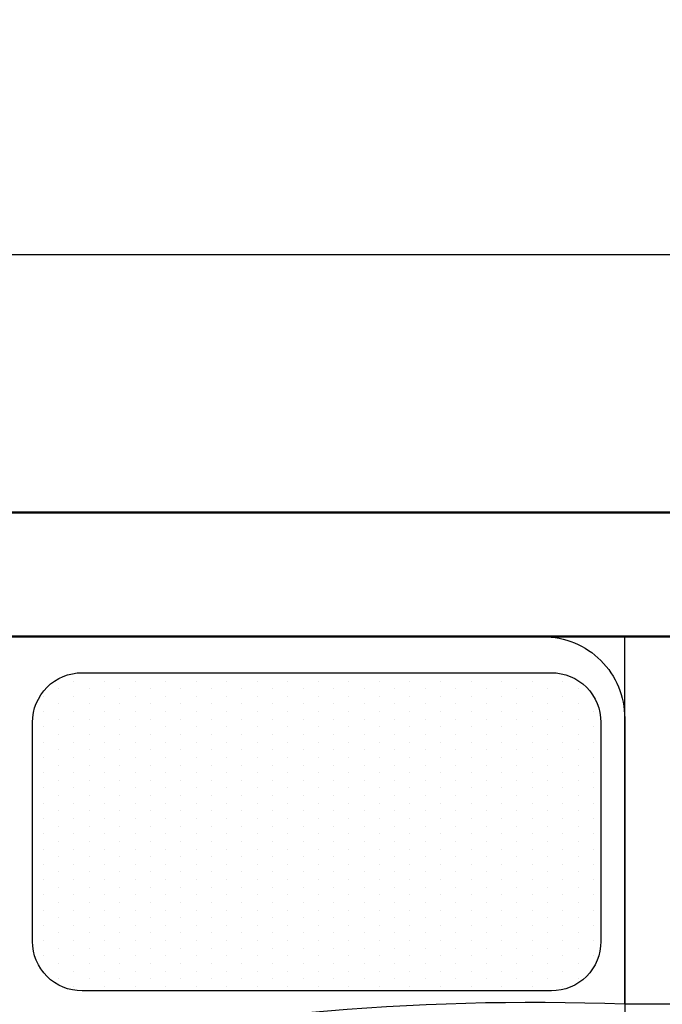
# Model space of a CAD drawing. Units: inches. Extents: x 3064 to 19385, y 846 to 15425.
# Tile 23 of 108: x 3886 to 3917, y 1373 to 1420. Entities that reach past the tile are written whole.
import ezdxf

# ---------------------------------------------------------------- set-up
doc = ezdxf.new("R2010")
doc.units = ezdxf.units.IN
for name, color, linetype, lineweight in [('A-ANNO-DIMS', 2, 'Continuous', 18), ('A-FLOR-FIXT', 9, 'Continuous', 18), ('A-WALL', 7, 'Continuous', 50)]:
    doc.layers.add(name, color=color, linetype=linetype, lineweight=lineweight)
doc.layers.add('BLOCK', color=6, linetype='Continuous')
doc.styles.get("Standard").update_dxf_attribs({"font": 'arial.ttf'})
doc.dimstyles.new('ISO-25', dxfattribs={"dimtxt": 9, "dimasz": 2.5, "dimexe": 1.25, "dimexo": 0.625, "dimtad": 1, "dimdec": 1, "dimlunit": 3, "dimtxsty": 'Standard', "dimcen": 2.5, "dimadec": 0, "dimazin": 0, "dimtfac": 1, "dimtdec": 1, "dimtmove": 0, "dimatfit": 3, "dimfxl": 1, "dimarcsym": 0})

# ---------------------------------------------------------------- blocks, each defined once
blk = doc.blocks.new('*X7')
at = {"color": 0}
for p, q in [((273.9375, 457.03125), (273.9375, 457.03125)), ((274.3125, 457.03125), (274.3125, 457.03125)), ((274.6875, 457.03125), (274.6875, 457.03125)), ((275.0625, 457.03125), (275.0625, 457.03125)), ((275.4375, 457.03125), (275.4375, 457.03125)), ((275.8125, 457.03125), (275.8125, 457.03125)), ((276.1875, 457.03125), (276.1875, 457.03125)), ((276.5625, 457.03125), (276.5625, 457.03125)), ((276.9375, 457.03125), (276.9375, 457.03125)), ((277.3125, 457.03125), (277.3125, 457.03125)), ((277.6875, 457.03125), (277.6875, 457.03125)), ((278.0625, 457.03125), (278.0625, 457.03125)), ((278.4375, 457.03125), (278.4375, 457.03125)), ((278.8125, 457.03125), (278.8125, 457.03125)), ((279.1875, 457.03125), (279.1875, 457.03125)), ((279.5625, 457.03125), (279.5625, 457.03125)), ((273.5625, 456.84375), (273.5625, 456.84375)), ((273.75, 456.9375), (273.75, 456.9375)), ((273.9375, 456.84375), (273.9375, 456.84375)), ((274.125, 456.9375), (274.125, 456.9375)), ((274.3125, 456.84375), (274.3125, 456.84375)), ((274.5, 456.9375), (274.5, 456.9375)), ((274.6875, 456.84375), (274.6875, 456.84375)), ((274.875, 456.9375), (274.875, 456.9375)), ((275.0625, 456.84375), (275.0625, 456.84375)), ((275.25, 456.9375), (275.25, 456.9375)), ((275.4375, 456.84375), (275.4375, 456.84375)), ((275.625, 456.9375), (275.625, 456.9375)), ((275.8125, 456.84375), (275.8125, 456.84375)), ((276, 456.9375), (276, 456.9375)), ((276.1875, 456.84375), (276.1875, 456.84375)), ((276.375, 456.9375), (276.375, 456.9375)), ((276.5625, 456.84375), (276.5625, 456.84375)), ((276.75, 456.9375), (276.75, 456.9375)), ((276.9375, 456.84375), (276.9375, 456.84375)), ((277.125, 456.9375), (277.125, 456.9375)), ((277.3125, 456.84375), (277.3125, 456.84375)), ((277.5, 456.9375), (277.5, 456.9375)), ((277.6875, 456.84375), (277.6875, 456.84375)), ((277.875, 456.9375), (277.875, 456.9375)), ((278.0625, 456.84375), (278.0625, 456.84375)), ((278.25, 456.9375), (278.25, 456.9375)), ((278.4375, 456.84375), (278.4375, 456.84375)), ((278.625, 456.9375), (278.625, 456.9375)), ((278.8125, 456.84375), (278.8125, 456.84375)), ((279, 456.9375), (279, 456.9375)), ((279.1875, 456.84375), (279.1875, 456.84375)), ((279.375, 456.9375), (279.375, 456.9375)), ((279.5625, 456.84375), (279.5625, 456.84375)), ((279.75, 456.9375), (279.75, 456.9375)), ((279.9375, 456.84375), (279.9375, 456.84375)), ((273.375, 456.75), (273.375, 456.75)), ((273.75, 456.75), (273.75, 456.75)), ((274.125, 456.75), (274.125, 456.75)), ((274.5, 456.75), (274.5, 456.75)), ((274.875, 456.75), (274.875, 456.75)), ((275.25, 456.75), (275.25, 456.75)), ((275.625, 456.75), (275.625, 456.75)), ((276, 456.75), (276, 456.75)), ((276.375, 456.75), (276.375, 456.75)), ((276.75, 456.75), (276.75, 456.75)), ((277.125, 456.75), (277.125, 456.75)), ((277.5, 456.75), (277.5, 456.75)), ((277.875, 456.75), (277.875, 456.75)), ((278.25, 456.75), (278.25, 456.75)), ((278.625, 456.75), (278.625, 456.75)), ((279, 456.75), (279, 456.75)), ((279.375, 456.75), (279.375, 456.75)), ((279.75, 456.75), (279.75, 456.75)), ((280.125, 456.75), (280.125, 456.75)), ((273.5625, 456.65625), (273.5625, 456.65625)), ((273.9375, 456.65625), (273.9375, 456.65625)), ((274.3125, 456.65625), (274.3125, 456.65625)), ((274.6875, 456.65625), (274.6875, 456.65625)), ((275.0625, 456.65625), (275.0625, 456.65625)), ((275.4375, 456.65625), (275.4375, 456.65625)), ((275.8125, 456.65625), (275.8125, 456.65625)), ((276.1875, 456.65625), (276.1875, 456.65625)), ((276.5625, 456.65625), (276.5625, 456.65625)), ((276.9375, 456.65625), (276.9375, 456.65625)), ((277.3125, 456.65625), (277.3125, 456.65625)), ((277.6875, 456.65625), (277.6875, 456.65625)), ((278.0625, 456.65625), (278.0625, 456.65625)), ((278.4375, 456.65625), (278.4375, 456.65625)), ((278.8125, 456.65625), (278.8125, 456.65625)), ((279.1875, 456.65625), (279.1875, 456.65625)), ((279.5625, 456.65625), (279.5625, 456.65625)), ((279.9375, 456.65625), (279.9375, 456.65625)), ((273.375, 456.5625), (273.375, 456.5625)), ((273.75, 456.5625), (273.75, 456.5625)), ((274.125, 456.5625), (274.125, 456.5625)), ((274.5, 456.5625), (274.5, 456.5625)), ((274.875, 456.5625), (274.875, 456.5625)), ((275.25, 456.5625), (275.25, 456.5625)), ((275.625, 456.5625), (275.625, 456.5625)), ((276, 456.5625), (276, 456.5625)), ((276.375, 456.5625), (276.375, 456.5625)), ((276.75, 456.5625), (276.75, 456.5625)), ((277.125, 456.5625), (277.125, 456.5625)), ((277.5, 456.5625), (277.5, 456.5625)), ((277.875, 456.5625), (277.875, 456.5625)), ((278.25, 456.5625), (278.25, 456.5625)), ((278.625, 456.5625), (278.625, 456.5625)), ((279, 456.5625), (279, 456.5625)), ((279.375, 456.5625), (279.375, 456.5625)), ((279.75, 456.5625), (279.75, 456.5625)), ((280.125, 456.5625), (280.125, 456.5625)), ((273.375, 456.375), (273.375, 456.375)), ((273.5625, 456.46875), (273.5625, 456.46875)), ((273.75, 456.375), (273.75, 456.375)), ((273.9375, 456.46875), (273.9375, 456.46875)), ((274.125, 456.375), (274.125, 456.375)), ((274.3125, 456.46875), (274.3125, 456.46875)), ((274.5, 456.375), (274.5, 456.375)), ((274.6875, 456.46875), (274.6875, 456.46875)), ((274.875, 456.375), (274.875, 456.375)), ((275.0625, 456.46875), (275.0625, 456.46875)), ((275.25, 456.375), (275.25, 456.375)), ((275.4375, 456.46875), (275.4375, 456.46875)), ((275.625, 456.375), (275.625, 456.375)), ((275.8125, 456.46875), (275.8125, 456.46875)), ((276, 456.375), (276, 456.375)), ((276.1875, 456.46875), (276.1875, 456.46875)), ((276.375, 456.375), (276.375, 456.375)), ((276.5625, 456.46875), (276.5625, 456.46875)), ((276.75, 456.375), (276.75, 456.375)), ((276.9375, 456.46875), (276.9375, 456.46875)), ((277.125, 456.375), (277.125, 456.375)), ((277.3125, 456.46875), (277.3125, 456.46875)), ((277.5, 456.375), (277.5, 456.375)), ((277.6875, 456.46875), (277.6875, 456.46875)), ((277.875, 456.375), (277.875, 456.375)), ((278.0625, 456.46875), (278.0625, 456.46875)), ((278.25, 456.375), (278.25, 456.375)), ((278.4375, 456.46875), (278.4375, 456.46875)), ((278.625, 456.375), (278.625, 456.375)), ((278.8125, 456.46875), (278.8125, 456.46875)), ((279, 456.375), (279, 456.375)), ((279.1875, 456.46875), (279.1875, 456.46875)), ((279.375, 456.375), (279.375, 456.375)), ((279.5625, 456.46875), (279.5625, 456.46875)), ((279.75, 456.375), (279.75, 456.375)), ((279.9375, 456.46875), (279.9375, 456.46875)), ((280.125, 456.375), (280.125, 456.375)), ((273.5625, 456.28125), (273.5625, 456.28125)), ((273.9375, 456.28125), (273.9375, 456.28125)), ((274.3125, 456.28125), (274.3125, 456.28125)), ((274.6875, 456.28125), (274.6875, 456.28125)), ((275.0625, 456.28125), (275.0625, 456.28125)), ((275.4375, 456.28125), (275.4375, 456.28125)), ((275.8125, 456.28125), (275.8125, 456.28125)), ((276.1875, 456.28125), (276.1875, 456.28125)), ((276.5625, 456.28125), (276.5625, 456.28125)), ((276.9375, 456.28125), (276.9375, 456.28125)), ((277.3125, 456.28125), (277.3125, 456.28125)), ((277.6875, 456.28125), (277.6875, 456.28125)), ((278.0625, 456.28125), (278.0625, 456.28125)), ((278.4375, 456.28125), (278.4375, 456.28125)), ((278.8125, 456.28125), (278.8125, 456.28125)), ((279.1875, 456.28125), (279.1875, 456.28125)), ((279.5625, 456.28125), (279.5625, 456.28125)), ((279.9375, 456.28125), (279.9375, 456.28125)), ((273.375, 456.1875), (273.375, 456.1875)), ((273.75, 456.1875), (273.75, 456.1875)), ((274.125, 456.1875), (274.125, 456.1875)), ((274.5, 456.1875), (274.5, 456.1875)), ((274.875, 456.1875), (274.875, 456.1875)), ((275.25, 456.1875), (275.25, 456.1875)), ((275.625, 456.1875), (275.625, 456.1875)), ((276, 456.1875), (276, 456.1875)), ((276.375, 456.1875), (276.375, 456.1875)), ((276.75, 456.1875), (276.75, 456.1875)), ((277.125, 456.1875), (277.125, 456.1875)), ((277.5, 456.1875), (277.5, 456.1875)), ((277.875, 456.1875), (277.875, 456.1875)), ((278.25, 456.1875), (278.25, 456.1875)), ((278.625, 456.1875), (278.625, 456.1875)), ((279, 456.1875), (279, 456.1875)), ((279.375, 456.1875), (279.375, 456.1875)), ((279.75, 456.1875), (279.75, 456.1875)), ((280.125, 456.1875), (280.125, 456.1875)), ((273.375, 456), (273.375, 456)), ((273.5625, 456.09375), (273.5625, 456.09375)), ((273.75, 456), (273.75, 456)), ((273.9375, 456.09375), (273.9375, 456.09375)), ((274.125, 456), (274.125, 456)), ((274.3125, 456.09375), (274.3125, 456.09375)), ((274.5, 456), (274.5, 456)), ((274.6875, 456.09375), (274.6875, 456.09375)), ((274.875, 456), (274.875, 456)), ((275.0625, 456.09375), (275.0625, 456.09375)), ((275.25, 456), (275.25, 456)), ((275.4375, 456.09375), (275.4375, 456.09375)), ((275.625, 456), (275.625, 456)), ((275.8125, 456.09375), (275.8125, 456.09375)), ((276, 456), (276, 456)), ((276.1875, 456.09375), (276.1875, 456.09375)), ((276.375, 456), (276.375, 456)), ((276.5625, 456.09375), (276.5625, 456.09375)), ((276.75, 456), (276.75, 456)), ((276.9375, 456.09375), (276.9375, 456.09375)), ((277.125, 456), (277.125, 456)), ((277.3125, 456.09375), (277.3125, 456.09375)), ((277.5, 456), (277.5, 456)), ((277.6875, 456.09375), (277.6875, 456.09375)), ((277.875, 456), (277.875, 456)), ((278.0625, 456.09375), (278.0625, 456.09375)), ((278.25, 456), (278.25, 456)), ((278.4375, 456.09375), (278.4375, 456.09375)), ((278.625, 456), (278.625, 456)), ((278.8125, 456.09375), (278.8125, 456.09375)), ((279, 456), (279, 456)), ((279.1875, 456.09375), (279.1875, 456.09375)), ((279.375, 456), (279.375, 456)), ((279.5625, 456.09375), (279.5625, 456.09375)), ((279.75, 456), (279.75, 456)), ((279.9375, 456.09375), (279.9375, 456.09375)), ((280.125, 456), (280.125, 456)), ((273.5625, 455.90625), (273.5625, 455.90625)), ((273.9375, 455.90625), (273.9375, 455.90625)), ((274.3125, 455.90625), (274.3125, 455.90625)), ((274.6875, 455.90625), (274.6875, 455.90625)), ((275.0625, 455.90625), (275.0625, 455.90625)), ((275.4375, 455.90625), (275.4375, 455.90625)), ((275.8125, 455.90625), (275.8125, 455.90625)), ((276.1875, 455.90625), (276.1875, 455.90625)), ((276.5625, 455.90625), (276.5625, 455.90625)), ((276.9375, 455.90625), (276.9375, 455.90625)), ((277.3125, 455.90625), (277.3125, 455.90625)), ((277.6875, 455.90625), (277.6875, 455.90625)), ((278.0625, 455.90625), (278.0625, 455.90625)), ((278.4375, 455.90625), (278.4375, 455.90625)), ((278.8125, 455.90625), (278.8125, 455.90625)), ((279.1875, 455.90625), (279.1875, 455.90625)), ((279.5625, 455.90625), (279.5625, 455.90625)), ((279.9375, 455.90625), (279.9375, 455.90625)), ((273.375, 455.8125), (273.375, 455.8125)), ((273.75, 455.8125), (273.75, 455.8125)), ((274.125, 455.8125), (274.125, 455.8125)), ((274.5, 455.8125), (274.5, 455.8125)), ((274.875, 455.8125), (274.875, 455.8125)), ((275.25, 455.8125), (275.25, 455.8125)), ((275.625, 455.8125), (275.625, 455.8125)), ((276, 455.8125), (276, 455.8125)), ((276.375, 455.8125), (276.375, 455.8125)), ((276.75, 455.8125), (276.75, 455.8125)), ((277.125, 455.8125), (277.125, 455.8125)), ((277.5, 455.8125), (277.5, 455.8125)), ((277.875, 455.8125), (277.875, 455.8125)), ((278.25, 455.8125), (278.25, 455.8125)), ((278.625, 455.8125), (278.625, 455.8125)), ((279, 455.8125), (279, 455.8125)), ((279.375, 455.8125), (279.375, 455.8125)), ((279.75, 455.8125), (279.75, 455.8125)), ((280.125, 455.8125), (280.125, 455.8125)), ((273.375, 455.625), (273.375, 455.625)), ((273.5625, 455.71875), (273.5625, 455.71875)), ((273.75, 455.625), (273.75, 455.625)), ((273.9375, 455.71875), (273.9375, 455.71875)), ((274.125, 455.625), (274.125, 455.625)), ((274.3125, 455.71875), (274.3125, 455.71875)), ((274.5, 455.625), (274.5, 455.625)), ((274.6875, 455.71875), (274.6875, 455.71875)), ((274.875, 455.625), (274.875, 455.625)), ((275.0625, 455.71875), (275.0625, 455.71875)), ((275.25, 455.625), (275.25, 455.625)), ((275.4375, 455.71875), (275.4375, 455.71875)), ((275.625, 455.625), (275.625, 455.625)), ((275.8125, 455.71875), (275.8125, 455.71875)), ((276, 455.625), (276, 455.625)), ((276.1875, 455.71875), (276.1875, 455.71875)), ((276.375, 455.625), (276.375, 455.625)), ((276.5625, 455.71875), (276.5625, 455.71875)), ((276.75, 455.625), (276.75, 455.625)), ((276.9375, 455.71875), (276.9375, 455.71875)), ((277.125, 455.625), (277.125, 455.625)), ((277.3125, 455.71875), (277.3125, 455.71875)), ((277.5, 455.625), (277.5, 455.625)), ((277.6875, 455.71875), (277.6875, 455.71875)), ((277.875, 455.625), (277.875, 455.625)), ((278.0625, 455.71875), (278.0625, 455.71875)), ((278.25, 455.625), (278.25, 455.625)), ((278.4375, 455.71875), (278.4375, 455.71875)), ((278.625, 455.625), (278.625, 455.625)), ((278.8125, 455.71875), (278.8125, 455.71875)), ((279, 455.625), (279, 455.625)), ((279.1875, 455.71875), (279.1875, 455.71875)), ((279.375, 455.625), (279.375, 455.625)), ((279.5625, 455.71875), (279.5625, 455.71875)), ((279.75, 455.625), (279.75, 455.625)), ((279.9375, 455.71875), (279.9375, 455.71875)), ((280.125, 455.625), (280.125, 455.625)), ((273.5625, 455.53125), (273.5625, 455.53125)), ((273.9375, 455.53125), (273.9375, 455.53125)), ((274.3125, 455.53125), (274.3125, 455.53125)), ((274.6875, 455.53125), (274.6875, 455.53125)), ((275.0625, 455.53125), (275.0625, 455.53125)), ((275.4375, 455.53125), (275.4375, 455.53125)), ((275.8125, 455.53125), (275.8125, 455.53125)), ((276.1875, 455.53125), (276.1875, 455.53125)), ((276.5625, 455.53125), (276.5625, 455.53125)), ((276.9375, 455.53125), (276.9375, 455.53125)), ((277.3125, 455.53125), (277.3125, 455.53125)), ((277.6875, 455.53125), (277.6875, 455.53125)), ((278.0625, 455.53125), (278.0625, 455.53125)), ((278.4375, 455.53125), (278.4375, 455.53125)), ((278.8125, 455.53125), (278.8125, 455.53125)), ((279.1875, 455.53125), (279.1875, 455.53125)), ((279.5625, 455.53125), (279.5625, 455.53125)), ((279.9375, 455.53125), (279.9375, 455.53125)), ((273.375, 455.4375), (273.375, 455.4375)), ((273.75, 455.4375), (273.75, 455.4375)), ((274.125, 455.4375), (274.125, 455.4375)), ((274.5, 455.4375), (274.5, 455.4375)), ((274.875, 455.4375), (274.875, 455.4375)), ((275.25, 455.4375), (275.25, 455.4375)), ((275.625, 455.4375), (275.625, 455.4375)), ((276, 455.4375), (276, 455.4375)), ((276.375, 455.4375), (276.375, 455.4375)), ((276.75, 455.4375), (276.75, 455.4375)), ((277.125, 455.4375), (277.125, 455.4375)), ((277.5, 455.4375), (277.5, 455.4375)), ((277.875, 455.4375), (277.875, 455.4375)), ((278.25, 455.4375), (278.25, 455.4375)), ((278.625, 455.4375), (278.625, 455.4375)), ((279, 455.4375), (279, 455.4375)), ((279.375, 455.4375), (279.375, 455.4375)), ((279.75, 455.4375), (279.75, 455.4375)), ((280.125, 455.4375), (280.125, 455.4375)), ((273.5625, 455.34375), (273.5625, 455.34375)), ((273.9375, 455.34375), (273.9375, 455.34375)), ((274.3125, 455.34375), (274.3125, 455.34375)), ((274.6875, 455.34375), (274.6875, 455.34375)), ((275.0625, 455.34375), (275.0625, 455.34375)), ((275.4375, 455.34375), (275.4375, 455.34375)), ((275.8125, 455.34375), (275.8125, 455.34375)), ((276.1875, 455.34375), (276.1875, 455.34375)), ((276.5625, 455.34375), (276.5625, 455.34375)), ((276.9375, 455.34375), (276.9375, 455.34375)), ((277.3125, 455.34375), (277.3125, 455.34375)), ((277.6875, 455.34375), (277.6875, 455.34375)), ((278.0625, 455.34375), (278.0625, 455.34375)), ((278.4375, 455.34375), (278.4375, 455.34375)), ((278.8125, 455.34375), (278.8125, 455.34375)), ((279.1875, 455.34375), (279.1875, 455.34375)), ((279.5625, 455.34375), (279.5625, 455.34375)), ((279.9375, 455.34375), (279.9375, 455.34375)), ((273.375, 455.25), (273.375, 455.25)), ((273.5625, 455.15625), (273.5625, 455.15625)), ((273.75, 455.25), (273.75, 455.25)), ((273.9375, 455.15625), (273.9375, 455.15625)), ((274.125, 455.25), (274.125, 455.25)), ((274.3125, 455.15625), (274.3125, 455.15625)), ((274.5, 455.25), (274.5, 455.25)), ((274.6875, 455.15625), (274.6875, 455.15625)), ((274.875, 455.25), (274.875, 455.25)), ((275.0625, 455.15625), (275.0625, 455.15625)), ((275.25, 455.25), (275.25, 455.25)), ((275.4375, 455.15625), (275.4375, 455.15625)), ((275.625, 455.25), (275.625, 455.25)), ((275.8125, 455.15625), (275.8125, 455.15625)), ((276, 455.25), (276, 455.25)), ((276.1875, 455.15625), (276.1875, 455.15625)), ((276.375, 455.25), (276.375, 455.25)), ((276.5625, 455.15625), (276.5625, 455.15625)), ((276.75, 455.25), (276.75, 455.25)), ((276.9375, 455.15625), (276.9375, 455.15625)), ((277.125, 455.25), (277.125, 455.25)), ((277.3125, 455.15625), (277.3125, 455.15625)), ((277.5, 455.25), (277.5, 455.25)), ((277.6875, 455.15625), (277.6875, 455.15625)), ((277.875, 455.25), (277.875, 455.25)), ((278.0625, 455.15625), (278.0625, 455.15625)), ((278.25, 455.25), (278.25, 455.25)), ((278.4375, 455.15625), (278.4375, 455.15625)), ((278.625, 455.25), (278.625, 455.25)), ((278.8125, 455.15625), (278.8125, 455.15625)), ((279, 455.25), (279, 455.25)), ((279.1875, 455.15625), (279.1875, 455.15625)), ((279.375, 455.25), (279.375, 455.25)), ((279.5625, 455.15625), (279.5625, 455.15625)), ((279.75, 455.25), (279.75, 455.25)), ((279.9375, 455.15625), (279.9375, 455.15625)), ((280.125, 455.25), (280.125, 455.25)), ((273.375, 455.0625), (273.375, 455.0625)), ((273.75, 455.0625), (273.75, 455.0625)), ((274.125, 455.0625), (274.125, 455.0625)), ((274.5, 455.0625), (274.5, 455.0625)), ((274.875, 455.0625), (274.875, 455.0625)), ((275.25, 455.0625), (275.25, 455.0625)), ((275.625, 455.0625), (275.625, 455.0625)), ((276, 455.0625), (276, 455.0625)), ((276.375, 455.0625), (276.375, 455.0625)), ((276.75, 455.0625), (276.75, 455.0625)), ((277.125, 455.0625), (277.125, 455.0625)), ((277.5, 455.0625), (277.5, 455.0625)), ((277.875, 455.0625), (277.875, 455.0625)), ((278.25, 455.0625), (278.25, 455.0625)), ((278.625, 455.0625), (278.625, 455.0625)), ((279, 455.0625), (279, 455.0625)), ((279.375, 455.0625), (279.375, 455.0625)), ((279.75, 455.0625), (279.75, 455.0625)), ((280.125, 455.0625), (280.125, 455.0625)), ((273.5625, 454.96875), (273.5625, 454.96875)), ((273.9375, 454.96875), (273.9375, 454.96875)), ((274.3125, 454.96875), (274.3125, 454.96875)), ((274.6875, 454.96875), (274.6875, 454.96875)), ((275.0625, 454.96875), (275.0625, 454.96875)), ((275.4375, 454.96875), (275.4375, 454.96875)), ((275.8125, 454.96875), (275.8125, 454.96875)), ((276.1875, 454.96875), (276.1875, 454.96875)), ((276.5625, 454.96875), (276.5625, 454.96875)), ((276.9375, 454.96875), (276.9375, 454.96875)), ((277.3125, 454.96875), (277.3125, 454.96875)), ((277.6875, 454.96875), (277.6875, 454.96875)), ((278.0625, 454.96875), (278.0625, 454.96875)), ((278.4375, 454.96875), (278.4375, 454.96875)), ((278.8125, 454.96875), (278.8125, 454.96875)), ((279.1875, 454.96875), (279.1875, 454.96875)), ((279.5625, 454.96875), (279.5625, 454.96875)), ((279.9375, 454.96875), (279.9375, 454.96875)), ((273.375, 454.875), (273.375, 454.875)), ((273.5625, 454.78125), (273.5625, 454.78125)), ((273.75, 454.875), (273.75, 454.875)), ((273.9375, 454.78125), (273.9375, 454.78125)), ((274.125, 454.875), (274.125, 454.875)), ((274.3125, 454.78125), (274.3125, 454.78125)), ((274.5, 454.875), (274.5, 454.875)), ((274.6875, 454.78125), (274.6875, 454.78125)), ((274.875, 454.875), (274.875, 454.875)), ((275.0625, 454.78125), (275.0625, 454.78125)), ((275.25, 454.875), (275.25, 454.875)), ((275.4375, 454.78125), (275.4375, 454.78125)), ((275.625, 454.875), (275.625, 454.875)), ((275.8125, 454.78125), (275.8125, 454.78125)), ((276, 454.875), (276, 454.875)), ((276.1875, 454.78125), (276.1875, 454.78125)), ((276.375, 454.875), (276.375, 454.875)), ((276.5625, 454.78125), (276.5625, 454.78125)), ((276.75, 454.875), (276.75, 454.875)), ((276.9375, 454.78125), (276.9375, 454.78125)), ((277.125, 454.875), (277.125, 454.875)), ((277.3125, 454.78125), (277.3125, 454.78125)), ((277.5, 454.875), (277.5, 454.875)), ((277.6875, 454.78125), (277.6875, 454.78125)), ((277.875, 454.875), (277.875, 454.875)), ((278.0625, 454.78125), (278.0625, 454.78125)), ((278.25, 454.875), (278.25, 454.875)), ((278.4375, 454.78125), (278.4375, 454.78125)), ((278.625, 454.875), (278.625, 454.875)), ((278.8125, 454.78125), (278.8125, 454.78125)), ((279, 454.875), (279, 454.875)), ((279.1875, 454.78125), (279.1875, 454.78125)), ((279.375, 454.875), (279.375, 454.875)), ((279.5625, 454.78125), (279.5625, 454.78125)), ((279.75, 454.875), (279.75, 454.875)), ((279.9375, 454.78125), (279.9375, 454.78125)), ((280.125, 454.875), (280.125, 454.875)), ((273.375, 454.6875), (273.375, 454.6875)), ((273.75, 454.6875), (273.75, 454.6875)), ((274.125, 454.6875), (274.125, 454.6875)), ((274.5, 454.6875), (274.5, 454.6875)), ((274.875, 454.6875), (274.875, 454.6875)), ((275.25, 454.6875), (275.25, 454.6875)), ((275.625, 454.6875), (275.625, 454.6875)), ((276, 454.6875), (276, 454.6875)), ((276.375, 454.6875), (276.375, 454.6875)), ((276.75, 454.6875), (276.75, 454.6875)), ((277.125, 454.6875), (277.125, 454.6875)), ((277.5, 454.6875), (277.5, 454.6875)), ((277.875, 454.6875), (277.875, 454.6875)), ((278.25, 454.6875), (278.25, 454.6875)), ((278.625, 454.6875), (278.625, 454.6875)), ((279, 454.6875), (279, 454.6875)), ((279.375, 454.6875), (279.375, 454.6875)), ((279.75, 454.6875), (279.75, 454.6875)), ((280.125, 454.6875), (280.125, 454.6875)), ((273.5625, 454.59375), (273.5625, 454.59375)), ((273.9375, 454.59375), (273.9375, 454.59375)), ((274.3125, 454.59375), (274.3125, 454.59375)), ((274.6875, 454.59375), (274.6875, 454.59375)), ((275.0625, 454.59375), (275.0625, 454.59375)), ((275.4375, 454.59375), (275.4375, 454.59375)), ((275.8125, 454.59375), (275.8125, 454.59375)), ((276.1875, 454.59375), (276.1875, 454.59375)), ((276.5625, 454.59375), (276.5625, 454.59375)), ((276.9375, 454.59375), (276.9375, 454.59375)), ((277.3125, 454.59375), (277.3125, 454.59375)), ((277.6875, 454.59375), (277.6875, 454.59375)), ((278.0625, 454.59375), (278.0625, 454.59375)), ((278.4375, 454.59375), (278.4375, 454.59375)), ((278.8125, 454.59375), (278.8125, 454.59375)), ((279.1875, 454.59375), (279.1875, 454.59375)), ((279.5625, 454.59375), (279.5625, 454.59375)), ((279.9375, 454.59375), (279.9375, 454.59375)), ((273.375, 454.5), (273.375, 454.5)), ((273.75, 454.5), (273.75, 454.5)), ((274.125, 454.5), (274.125, 454.5)), ((274.5, 454.5), (274.5, 454.5)), ((274.875, 454.5), (274.875, 454.5)), ((275.25, 454.5), (275.25, 454.5)), ((275.625, 454.5), (275.625, 454.5)), ((276, 454.5), (276, 454.5)), ((276.375, 454.5), (276.375, 454.5)), ((276.75, 454.5), (276.75, 454.5)), ((277.125, 454.5), (277.125, 454.5)), ((277.5, 454.5), (277.5, 454.5)), ((277.875, 454.5), (277.875, 454.5)), ((278.25, 454.5), (278.25, 454.5)), ((278.625, 454.5), (278.625, 454.5)), ((279, 454.5), (279, 454.5)), ((279.375, 454.5), (279.375, 454.5)), ((279.75, 454.5), (279.75, 454.5)), ((280.125, 454.5), (280.125, 454.5)), ((273.375, 454.3125), (273.375, 454.3125)), ((273.5625, 454.40625), (273.5625, 454.40625)), ((273.75, 454.3125), (273.75, 454.3125)), ((273.9375, 454.40625), (273.9375, 454.40625)), ((274.125, 454.3125), (274.125, 454.3125)), ((274.3125, 454.40625), (274.3125, 454.40625)), ((274.5, 454.3125), (274.5, 454.3125)), ((274.6875, 454.40625), (274.6875, 454.40625)), ((274.875, 454.3125), (274.875, 454.3125)), ((275.0625, 454.40625), (275.0625, 454.40625)), ((275.25, 454.3125), (275.25, 454.3125)), ((275.4375, 454.40625), (275.4375, 454.40625)), ((275.625, 454.3125), (275.625, 454.3125)), ((275.8125, 454.40625), (275.8125, 454.40625)), ((276, 454.3125), (276, 454.3125)), ((276.1875, 454.40625), (276.1875, 454.40625)), ((276.375, 454.3125), (276.375, 454.3125)), ((276.5625, 454.40625), (276.5625, 454.40625)), ((276.75, 454.3125), (276.75, 454.3125)), ((276.9375, 454.40625), (276.9375, 454.40625)), ((277.125, 454.3125), (277.125, 454.3125)), ((277.3125, 454.40625), (277.3125, 454.40625)), ((277.5, 454.3125), (277.5, 454.3125)), ((277.6875, 454.40625), (277.6875, 454.40625)), ((277.875, 454.3125), (277.875, 454.3125)), ((278.0625, 454.40625), (278.0625, 454.40625)), ((278.25, 454.3125), (278.25, 454.3125)), ((278.4375, 454.40625), (278.4375, 454.40625)), ((278.625, 454.3125), (278.625, 454.3125)), ((278.8125, 454.40625), (278.8125, 454.40625)), ((279, 454.3125), (279, 454.3125)), ((279.1875, 454.40625), (279.1875, 454.40625)), ((279.375, 454.3125), (279.375, 454.3125)), ((279.5625, 454.40625), (279.5625, 454.40625)), ((279.75, 454.3125), (279.75, 454.3125)), ((279.9375, 454.40625), (279.9375, 454.40625)), ((280.125, 454.3125), (280.125, 454.3125)), ((273.5625, 454.21875), (273.5625, 454.21875)), ((273.9375, 454.21875), (273.9375, 454.21875)), ((274.3125, 454.21875), (274.3125, 454.21875)), ((274.6875, 454.21875), (274.6875, 454.21875)), ((275.0625, 454.21875), (275.0625, 454.21875)), ((275.4375, 454.21875), (275.4375, 454.21875)), ((275.8125, 454.21875), (275.8125, 454.21875)), ((276.1875, 454.21875), (276.1875, 454.21875)), ((276.5625, 454.21875), (276.5625, 454.21875)), ((276.9375, 454.21875), (276.9375, 454.21875)), ((277.3125, 454.21875), (277.3125, 454.21875)), ((277.6875, 454.21875), (277.6875, 454.21875)), ((278.0625, 454.21875), (278.0625, 454.21875)), ((278.4375, 454.21875), (278.4375, 454.21875)), ((278.8125, 454.21875), (278.8125, 454.21875)), ((279.1875, 454.21875), (279.1875, 454.21875)), ((279.5625, 454.21875), (279.5625, 454.21875)), ((279.9375, 454.21875), (279.9375, 454.21875)), ((273.375, 454.125), (273.375, 454.125)), ((273.75, 454.125), (273.75, 454.125)), ((274.125, 454.125), (274.125, 454.125)), ((274.5, 454.125), (274.5, 454.125)), ((274.875, 454.125), (274.875, 454.125)), ((275.25, 454.125), (275.25, 454.125)), ((275.625, 454.125), (275.625, 454.125)), ((276, 454.125), (276, 454.125)), ((276.375, 454.125), (276.375, 454.125)), ((276.75, 454.125), (276.75, 454.125)), ((277.125, 454.125), (277.125, 454.125)), ((277.5, 454.125), (277.5, 454.125)), ((277.875, 454.125), (277.875, 454.125)), ((278.25, 454.125), (278.25, 454.125)), ((278.625, 454.125), (278.625, 454.125)), ((279, 454.125), (279, 454.125)), ((279.375, 454.125), (279.375, 454.125)), ((279.75, 454.125), (279.75, 454.125)), ((280.125, 454.125), (280.125, 454.125)), ((273.375, 453.9375), (273.375, 453.9375)), ((273.5625, 454.03125), (273.5625, 454.03125)), ((273.75, 453.9375), (273.75, 453.9375)), ((273.9375, 454.03125), (273.9375, 454.03125)), ((274.125, 453.9375), (274.125, 453.9375)), ((274.3125, 454.03125), (274.3125, 454.03125)), ((274.5, 453.9375), (274.5, 453.9375)), ((274.6875, 454.03125), (274.6875, 454.03125)), ((274.875, 453.9375), (274.875, 453.9375)), ((275.0625, 454.03125), (275.0625, 454.03125)), ((275.25, 453.9375), (275.25, 453.9375)), ((275.4375, 454.03125), (275.4375, 454.03125)), ((275.625, 453.9375), (275.625, 453.9375)), ((275.8125, 454.03125), (275.8125, 454.03125)), ((276, 453.9375), (276, 453.9375)), ((276.1875, 454.03125), (276.1875, 454.03125)), ((276.375, 453.9375), (276.375, 453.9375)), ((276.5625, 454.03125), (276.5625, 454.03125)), ((276.75, 453.9375), (276.75, 453.9375)), ((276.9375, 454.03125), (276.9375, 454.03125)), ((277.125, 453.9375), (277.125, 453.9375)), ((277.3125, 454.03125), (277.3125, 454.03125)), ((277.5, 453.9375), (277.5, 453.9375)), ((277.6875, 454.03125), (277.6875, 454.03125)), ((277.875, 453.9375), (277.875, 453.9375)), ((278.0625, 454.03125), (278.0625, 454.03125)), ((278.25, 453.9375), (278.25, 453.9375)), ((278.4375, 454.03125), (278.4375, 454.03125)), ((278.625, 453.9375), (278.625, 453.9375)), ((278.8125, 454.03125), (278.8125, 454.03125)), ((279, 453.9375), (279, 453.9375)), ((279.1875, 454.03125), (279.1875, 454.03125)), ((279.375, 453.9375), (279.375, 453.9375)), ((279.5625, 454.03125), (279.5625, 454.03125)), ((279.75, 453.9375), (279.75, 453.9375)), ((279.9375, 454.03125), (279.9375, 454.03125)), ((280.125, 453.9375), (280.125, 453.9375)), ((273.5625, 453.84375), (273.5625, 453.84375)), ((273.9375, 453.84375), (273.9375, 453.84375)), ((274.3125, 453.84375), (274.3125, 453.84375)), ((274.6875, 453.84375), (274.6875, 453.84375)), ((275.0625, 453.84375), (275.0625, 453.84375)), ((275.4375, 453.84375), (275.4375, 453.84375)), ((275.8125, 453.84375), (275.8125, 453.84375)), ((276.1875, 453.84375), (276.1875, 453.84375)), ((276.5625, 453.84375), (276.5625, 453.84375)), ((276.9375, 453.84375), (276.9375, 453.84375)), ((277.3125, 453.84375), (277.3125, 453.84375)), ((277.6875, 453.84375), (277.6875, 453.84375)), ((278.0625, 453.84375), (278.0625, 453.84375)), ((278.4375, 453.84375), (278.4375, 453.84375)), ((278.8125, 453.84375), (278.8125, 453.84375)), ((279.1875, 453.84375), (279.1875, 453.84375)), ((279.5625, 453.84375), (279.5625, 453.84375)), ((279.9375, 453.84375), (279.9375, 453.84375)), ((273.375, 453.75), (273.375, 453.75)), ((273.75, 453.75), (273.75, 453.75)), ((274.125, 453.75), (274.125, 453.75)), ((274.5, 453.75), (274.5, 453.75)), ((274.875, 453.75), (274.875, 453.75)), ((275.25, 453.75), (275.25, 453.75)), ((275.625, 453.75), (275.625, 453.75)), ((276, 453.75), (276, 453.75)), ((276.375, 453.75), (276.375, 453.75)), ((276.75, 453.75), (276.75, 453.75)), ((277.125, 453.75), (277.125, 453.75)), ((277.5, 453.75), (277.5, 453.75)), ((277.875, 453.75), (277.875, 453.75)), ((278.25, 453.75), (278.25, 453.75)), ((278.625, 453.75), (278.625, 453.75)), ((279, 453.75), (279, 453.75)), ((279.375, 453.75), (279.375, 453.75)), ((279.75, 453.75), (279.75, 453.75)), ((280.125, 453.75), (280.125, 453.75)), ((273.5625, 453.65625), (273.5625, 453.65625)), ((273.9375, 453.65625), (273.9375, 453.65625)), ((274.3125, 453.65625), (274.3125, 453.65625)), ((274.6875, 453.65625), (274.6875, 453.65625)), ((275.0625, 453.65625), (275.0625, 453.65625)), ((275.4375, 453.65625), (275.4375, 453.65625)), ((275.8125, 453.65625), (275.8125, 453.65625)), ((276.1875, 453.65625), (276.1875, 453.65625)), ((276.5625, 453.65625), (276.5625, 453.65625)), ((276.9375, 453.65625), (276.9375, 453.65625)), ((277.3125, 453.65625), (277.3125, 453.65625)), ((277.6875, 453.65625), (277.6875, 453.65625)), ((278.0625, 453.65625), (278.0625, 453.65625)), ((278.4375, 453.65625), (278.4375, 453.65625)), ((278.8125, 453.65625), (278.8125, 453.65625)), ((279.1875, 453.65625), (279.1875, 453.65625)), ((279.5625, 453.65625), (279.5625, 453.65625)), ((279.9375, 453.65625), (279.9375, 453.65625)), ((273.375, 453.5625), (273.375, 453.5625)), ((273.5625, 453.46875), (273.5625, 453.46875)), ((273.75, 453.5625), (273.75, 453.5625)), ((273.9375, 453.46875), (273.9375, 453.46875)), ((274.125, 453.5625), (274.125, 453.5625)), ((274.3125, 453.46875), (274.3125, 453.46875)), ((274.5, 453.5625), (274.5, 453.5625)), ((274.6875, 453.46875), (274.6875, 453.46875)), ((274.875, 453.5625), (274.875, 453.5625)), ((275.0625, 453.46875), (275.0625, 453.46875)), ((275.25, 453.5625), (275.25, 453.5625)), ((275.4375, 453.46875), (275.4375, 453.46875)), ((275.625, 453.5625), (275.625, 453.5625)), ((275.8125, 453.46875), (275.8125, 453.46875)), ((276, 453.5625), (276, 453.5625)), ((276.1875, 453.46875), (276.1875, 453.46875)), ((276.375, 453.5625), (276.375, 453.5625)), ((276.5625, 453.46875), (276.5625, 453.46875)), ((276.75, 453.5625), (276.75, 453.5625)), ((276.9375, 453.46875), (276.9375, 453.46875)), ((277.125, 453.5625), (277.125, 453.5625)), ((277.3125, 453.46875), (277.3125, 453.46875)), ((277.5, 453.5625), (277.5, 453.5625)), ((277.6875, 453.46875), (277.6875, 453.46875)), ((277.875, 453.5625), (277.875, 453.5625)), ((278.0625, 453.46875), (278.0625, 453.46875)), ((278.25, 453.5625), (278.25, 453.5625)), ((278.4375, 453.46875), (278.4375, 453.46875)), ((278.625, 453.5625), (278.625, 453.5625)), ((278.8125, 453.46875), (278.8125, 453.46875)), ((279, 453.5625), (279, 453.5625)), ((279.1875, 453.46875), (279.1875, 453.46875)), ((279.375, 453.5625), (279.375, 453.5625)), ((279.5625, 453.46875), (279.5625, 453.46875)), ((279.75, 453.5625), (279.75, 453.5625)), ((279.9375, 453.46875), (279.9375, 453.46875)), ((280.125, 453.5625), (280.125, 453.5625)), ((273.375, 453.375), (273.375, 453.375)), ((273.75, 453.375), (273.75, 453.375)), ((274.125, 453.375), (274.125, 453.375)), ((274.5, 453.375), (274.5, 453.375)), ((274.875, 453.375), (274.875, 453.375)), ((275.25, 453.375), (275.25, 453.375)), ((275.625, 453.375), (275.625, 453.375)), ((276, 453.375), (276, 453.375)), ((276.375, 453.375), (276.375, 453.375)), ((276.75, 453.375), (276.75, 453.375)), ((277.125, 453.375), (277.125, 453.375)), ((277.5, 453.375), (277.5, 453.375)), ((277.875, 453.375), (277.875, 453.375)), ((278.25, 453.375), (278.25, 453.375)), ((278.625, 453.375), (278.625, 453.375)), ((279, 453.375), (279, 453.375)), ((279.375, 453.375), (279.375, 453.375)), ((279.75, 453.375), (279.75, 453.375)), ((273.5625, 453.28125), (273.5625, 453.28125)), ((273.9375, 453.28125), (273.9375, 453.28125)), ((274.3125, 453.28125), (274.3125, 453.28125)), ((274.6875, 453.28125), (274.6875, 453.28125)), ((275.0625, 453.28125), (275.0625, 453.28125)), ((275.4375, 453.28125), (275.4375, 453.28125)), ((275.8125, 453.28125), (275.8125, 453.28125)), ((276.1875, 453.28125), (276.1875, 453.28125)), ((276.5625, 453.28125), (276.5625, 453.28125)), ((276.9375, 453.28125), (276.9375, 453.28125)), ((277.3125, 453.28125), (277.3125, 453.28125)), ((277.6875, 453.28125), (277.6875, 453.28125)), ((278.0625, 453.28125), (278.0625, 453.28125)), ((278.4375, 453.28125), (278.4375, 453.28125)), ((278.8125, 453.28125), (278.8125, 453.28125)), ((279.1875, 453.28125), (279.1875, 453.28125)), ((279.5625, 453.28125), (279.5625, 453.28125)), ((279.9375, 453.28125), (279.9375, 453.28125)), ((273.75, 453.1875), (273.75, 453.1875)), ((274.125, 453.1875), (274.125, 453.1875)), ((274.5, 453.1875), (274.5, 453.1875)), ((274.875, 453.1875), (274.875, 453.1875)), ((275.25, 453.1875), (275.25, 453.1875)), ((275.625, 453.1875), (275.625, 453.1875)), ((276, 453.1875), (276, 453.1875)), ((276.375, 453.1875), (276.375, 453.1875)), ((276.75, 453.1875), (276.75, 453.1875)), ((277.125, 453.1875), (277.125, 453.1875)), ((277.5, 453.1875), (277.5, 453.1875)), ((277.875, 453.1875), (277.875, 453.1875)), ((278.25, 453.1875), (278.25, 453.1875)), ((278.625, 453.1875), (278.625, 453.1875)), ((279, 453.1875), (279, 453.1875)), ((279.375, 453.1875), (279.375, 453.1875)), ((279.75, 453.1875), (279.75, 453.1875))]:
    blk.add_line(p, q, dxfattribs=at)
blk = doc.blocks.new('A$C52E67D0D')
at = {"layer": 'BLOCK'}
for points in [[(1901, 0), (601, 0, -0.414214), (501, 100), (501, 1700, -0.414214), (601, 1800), (1901, 1800, -0.414214), (2001, 1700), (2001, 100, -0.414214)], [(1911, 1365.1), (1335, 1365.1, -0.414214), (1274.2, 1425.9), (1274.2, 1694.8, -0.414214), (1335, 1755.7), (1911, 1755.7, -0.414214), (1971.8, 1694.8), (1971.8, 1425.9, -0.414214)]]:
    blk.add_lwpolyline(points, format="xyb", close=True, dxfattribs=at)
blk.add_lwpolyline([(2001, 1348.6), (2001, 1799.6), (2502, 1799.6), (2502, 1348.6)], close=True, dxfattribs=at)
blk.add_arc((1888.6, -1664.5), 3015.3, 87.8642, 117.4001, dxfattribs=at)
at = {"layer": 'BLOCK', "xscale": 100, "yscale": 100, "zscale": 100}
blk.add_blockref('*X7', (-26050, -43948.2), dxfattribs=at)
blk = doc.blocks.new('*D41')
at = {"layer": 'A-ANNO-DIMS', "color": 0, "lineweight": -2, "transparency": 16777216}
for p, q in [((3647.359, 1396.965), (3647.359, 1410.06)), ((3989.359, 1396.965), (3989.359, 1410.06)), ((3649.859, 1408.81), (3986.859, 1408.81))]:
    blk.add_line(p, q, dxfattribs=at)
at = {"layer": 'A-ANNO-DIMS', "color": 0, "transparency": 16777216}
for points in [[(3649.859, 1409.226), (3649.859, 1408.393), (3647.359, 1408.81)], [(3986.859, 1409.226), (3986.859, 1408.393), (3989.359, 1408.81)]]:
    blk.add_solid(points, dxfattribs=at)
at = {"layer": 'Defpoints', "color": 0, "transparency": 16777216}
for p in [(3989.359, 1408.81), (3647.359, 1396.34), (3989.359, 1396.34)]:
    blk.add_point(p, dxfattribs=at)
at = {"layer": 'A-ANNO-DIMS', "color": 0, "transparency": 16777216, "insert": (3818.359, 1414.03), "char_height": 9, "attachment_point": 5}
blk.add_mtext('28\'-6"', dxfattribs=at)

msp = doc.modelspace()

# ---------------------------------------------------------------- linework, layer by layer
at = {"layer": 'A-WALL'}
for p, q in [((3989.359, 1396.34), (3647.359, 1396.34)), ((3983.359, 1390.34), (3788.359, 1390.34))]:
    msp.add_line(p, q, dxfattribs=at)

# ---------------------------------------------------------------- block references
at = {"layer": 'A-FLOR-FIXT', "xscale": 0.039370099999992, "yscale": 0.039370099999992, "zscale": 0.039370099999992}
msp.add_blockref('A$C52E67D0D', (3836.607, 1319.474), dxfattribs=at)

# ---------------------------------------------------------------- dimensions: what is measured, and where the dimension line sits
at = {"layer": 'A-ANNO-DIMS'}
dim = msp.add_linear_dim(base=(3989.359, 1408.81), p1=(3647.359, 1396.34), p2=(3989.359, 1396.34), dimstyle='ISO-25', override={"dimclrd": 0, "dimclre": 0, "dimclrt": 0}, dxfattribs=at)
dim.commit()
dim.dimension.update_dxf_attribs({"geometry": '*D41', "text_midpoint": (3818.359, 1414.03)})

doc.saveas('drawing.dxf')
